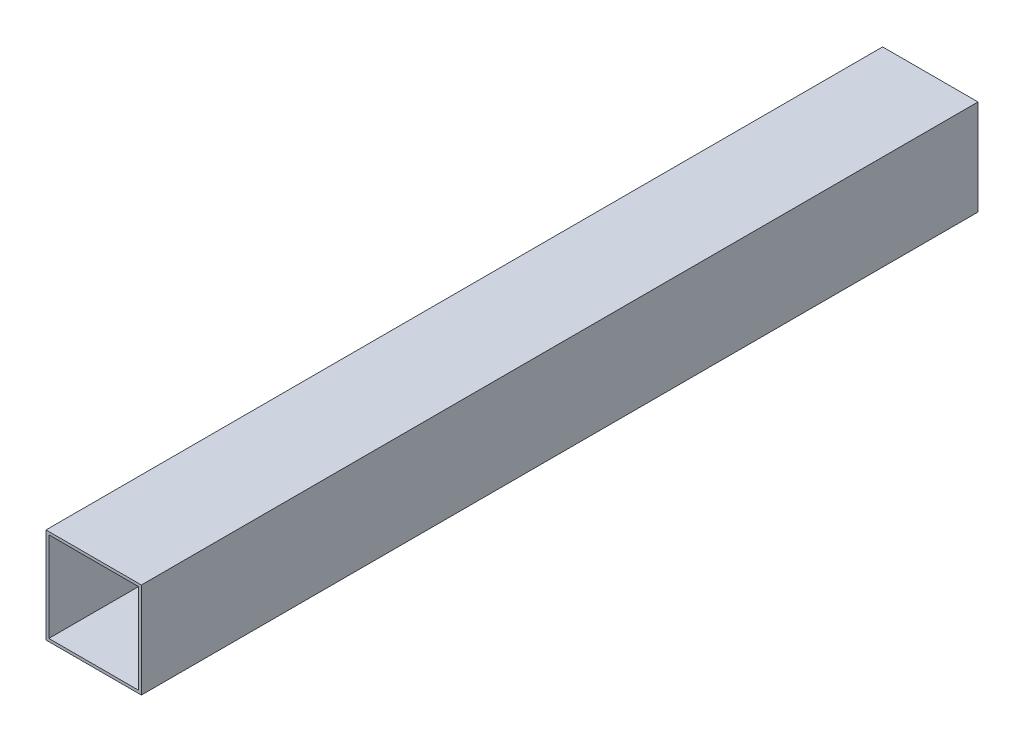
ISO-10303-21;
HEADER;
FILE_DESCRIPTION(('STEP AP214'),'2;1');
FILE_NAME('part.step','',(''),(''),'','','');
FILE_SCHEMA(('AUTOMOTIVE_DESIGN { 1 0 10303 214 1 1 1 1 }'));
ENDSEC;
DATA;
#1=APPLICATION_CONTEXT('core data for automotive mechanical design processes');
#2=APPLICATION_PROTOCOL_DEFINITION('international standard','automotive_design',2000,#1);
#3=PRODUCT_CONTEXT('',#1,'mechanical');
#4=PRODUCT('Part','Part','',(#3));
#5=PRODUCT_RELATED_PRODUCT_CATEGORY('part','',(#4));
#6=PRODUCT_DEFINITION_FORMATION('','',#4);
#7=PRODUCT_DEFINITION_CONTEXT('part definition',#1,'design');
#8=PRODUCT_DEFINITION('design','',#6,#7);
#9=PRODUCT_DEFINITION_SHAPE('','',#8);
#10=(LENGTH_UNIT() NAMED_UNIT(*) SI_UNIT(.MILLI.,.METRE.));
#11=(NAMED_UNIT(*) PLANE_ANGLE_UNIT() SI_UNIT($,.RADIAN.));
#12=(NAMED_UNIT(*) SI_UNIT($,.STERADIAN.) SOLID_ANGLE_UNIT());
#13=UNCERTAINTY_MEASURE_WITH_UNIT(LENGTH_MEASURE(1.E-05),#10,'distance_accuracy_value','');
#14=(GEOMETRIC_REPRESENTATION_CONTEXT(3) GLOBAL_UNCERTAINTY_ASSIGNED_CONTEXT((#13)) GLOBAL_UNIT_ASSIGNED_CONTEXT((#10,
#11,#12)) REPRESENTATION_CONTEXT('',''));
#15=CARTESIAN_POINT('',(0.,0.,0.));
#16=DIRECTION('',(0.,0.,1.));
#17=DIRECTION('',(1.,0.,0.));
#18=AXIS2_PLACEMENT_3D('',#15,#16,#17);
#19=CARTESIAN_POINT('',(0.,107.95,1893.8875));
#20=DIRECTION('',(0.,1.,0.));
#21=DIRECTION('',(0.,0.,1.));
#22=AXIS2_PLACEMENT_3D('',#19,#20,#21);
#23=PLANE('',#22);
#24=DIRECTION('',(1.,0.,0.));
#25=VECTOR('',#24,1.);
#26=CARTESIAN_POINT('',(0.,107.95,0.));
#27=LINE('',#26,#25);
#28=CARTESIAN_POINT('',(-107.95,107.95,0.));
#29=VERTEX_POINT('',#28);
#30=CARTESIAN_POINT('',(107.95,107.95,0.));
#31=VERTEX_POINT('',#30);
#32=EDGE_CURVE('E159',#29,#31,#27,.T.);
#33=ORIENTED_EDGE('',*,*,#32,.F.);
#34=DIRECTION('',(0.,0.,-1.));
#35=VECTOR('',#34,1.);
#36=CARTESIAN_POINT('',(-107.95,107.95,1893.8875));
#37=LINE('',#36,#35);
#38=CARTESIAN_POINT('',(-107.95,107.95,1893.8875));
#39=VERTEX_POINT('',#38);
#40=EDGE_CURVE('E12',#39,#29,#37,.T.);
#41=ORIENTED_EDGE('',*,*,#40,.F.);
#42=DIRECTION('',(1.,0.,0.));
#43=VECTOR('',#42,1.);
#44=CARTESIAN_POINT('',(0.,107.95,1893.8875));
#45=LINE('',#44,#43);
#46=CARTESIAN_POINT('',(107.95,107.95,1893.8875));
#47=VERTEX_POINT('',#46);
#48=EDGE_CURVE('E161',#39,#47,#45,.T.);
#49=ORIENTED_EDGE('',*,*,#48,.T.);
#50=DIRECTION('',(0.,0.,-1.));
#51=VECTOR('',#50,1.);
#52=CARTESIAN_POINT('',(107.95,107.95,1893.8875));
#53=LINE('',#52,#51);
#54=EDGE_CURVE('E67',#47,#31,#53,.T.);
#55=ORIENTED_EDGE('',*,*,#54,.T.);
#56=EDGE_LOOP('',(#33,#41,#49,#55));
#57=FACE_BOUND('',#56,.T.);
#58=ADVANCED_FACE('F61',(#57),#23,.T.);
#59=CARTESIAN_POINT('',(-107.95,0.,1893.8875));
#60=DIRECTION('',(1.,0.,0.));
#61=DIRECTION('',(0.,0.,-1.));
#62=AXIS2_PLACEMENT_3D('',#59,#60,#61);
#63=PLANE('',#62);
#64=DIRECTION('',(0.,-1.,0.));
#65=VECTOR('',#64,1.);
#66=CARTESIAN_POINT('',(-107.95,0.,0.));
#67=LINE('',#66,#65);
#68=CARTESIAN_POINT('',(-107.95,-107.95,0.));
#69=VERTEX_POINT('',#68);
#70=EDGE_CURVE('E167',#29,#69,#67,.T.);
#71=ORIENTED_EDGE('',*,*,#70,.T.);
#72=DIRECTION('',(0.,0.,-1.));
#73=VECTOR('',#72,1.);
#74=CARTESIAN_POINT('',(-107.95,-107.95,1893.8875));
#75=LINE('',#74,#73);
#76=CARTESIAN_POINT('',(-107.95,-107.95,1893.8875));
#77=VERTEX_POINT('',#76);
#78=EDGE_CURVE('E73',#77,#69,#75,.T.);
#79=ORIENTED_EDGE('',*,*,#78,.F.);
#80=DIRECTION('',(0.,-1.,0.));
#81=VECTOR('',#80,1.);
#82=CARTESIAN_POINT('',(-107.95,0.,1893.8875));
#83=LINE('',#82,#81);
#84=EDGE_CURVE('E175',#39,#77,#83,.T.);
#85=ORIENTED_EDGE('',*,*,#84,.F.);
#86=ORIENTED_EDGE('',*,*,#40,.T.);
#87=EDGE_LOOP('',(#71,#79,#85,#86));
#88=FACE_BOUND('',#87,.T.);
#89=ADVANCED_FACE('F197',(#88),#63,.F.);
#90=CARTESIAN_POINT('',(0.,-107.95,1893.8875));
#91=DIRECTION('',(0.,1.,0.));
#92=DIRECTION('',(0.,0.,1.));
#93=AXIS2_PLACEMENT_3D('',#90,#91,#92);
#94=PLANE('',#93);
#95=DIRECTION('',(1.,0.,0.));
#96=VECTOR('',#95,1.);
#97=CARTESIAN_POINT('',(0.,-107.95,0.));
#98=LINE('',#97,#96);
#99=CARTESIAN_POINT('',(107.95,-107.95,0.));
#100=VERTEX_POINT('',#99);
#101=EDGE_CURVE('E177',#69,#100,#98,.T.);
#102=ORIENTED_EDGE('',*,*,#101,.T.);
#103=DIRECTION('',(0.,0.,-1.));
#104=VECTOR('',#103,1.);
#105=CARTESIAN_POINT('',(107.95,-107.95,1893.8875));
#106=LINE('',#105,#104);
#107=CARTESIAN_POINT('',(107.95,-107.95,1893.8875));
#108=VERTEX_POINT('',#107);
#109=EDGE_CURVE('E182',#108,#100,#106,.T.);
#110=ORIENTED_EDGE('',*,*,#109,.F.);
#111=DIRECTION('',(1.,0.,0.));
#112=VECTOR('',#111,1.);
#113=CARTESIAN_POINT('',(0.,-107.95,1893.8875));
#114=LINE('',#113,#112);
#115=EDGE_CURVE('E169',#77,#108,#114,.T.);
#116=ORIENTED_EDGE('',*,*,#115,.F.);
#117=ORIENTED_EDGE('',*,*,#78,.T.);
#118=EDGE_LOOP('',(#102,#110,#116,#117));
#119=FACE_BOUND('',#118,.T.);
#120=ADVANCED_FACE('F201',(#119),#94,.F.);
#121=CARTESIAN_POINT('',(107.95,0.,1893.8875));
#122=DIRECTION('',(1.,0.,0.));
#123=DIRECTION('',(0.,1.,0.));
#124=AXIS2_PLACEMENT_3D('',#121,#122,#123);
#125=PLANE('',#124);
#126=DIRECTION('',(0.,-1.,0.));
#127=VECTOR('',#126,1.);
#128=CARTESIAN_POINT('',(107.95,0.,0.));
#129=LINE('',#128,#127);
#130=EDGE_CURVE('E176',#31,#100,#129,.T.);
#131=ORIENTED_EDGE('',*,*,#130,.F.);
#132=ORIENTED_EDGE('',*,*,#54,.F.);
#133=DIRECTION('',(0.,-1.,0.));
#134=VECTOR('',#133,1.);
#135=CARTESIAN_POINT('',(107.95,0.,1893.8875));
#136=LINE('',#135,#134);
#137=EDGE_CURVE('E168',#47,#108,#136,.T.);
#138=ORIENTED_EDGE('',*,*,#137,.T.);
#139=ORIENTED_EDGE('',*,*,#109,.T.);
#140=EDGE_LOOP('',(#131,#132,#138,#139));
#141=FACE_BOUND('',#140,.T.);
#142=ADVANCED_FACE('F195',(#141),#125,.T.);
#143=CARTESIAN_POINT('',(0.,0.,1893.8875));
#144=DIRECTION('',(0.,0.,-1.));
#145=DIRECTION('',(-1.,0.,0.));
#146=AXIS2_PLACEMENT_3D('',#143,#144,#145);
#147=PLANE('',#146);
#148=DIRECTION('',(0.,-1.,0.));
#149=VECTOR('',#148,1.);
#150=CARTESIAN_POINT('',(-101.6,101.6,1893.8875));
#151=LINE('',#150,#149);
#152=CARTESIAN_POINT('',(-101.6,101.6,1893.8875));
#153=VERTEX_POINT('',#152);
#154=CARTESIAN_POINT('',(-101.6,-101.6,1893.8875));
#155=VERTEX_POINT('',#154);
#156=EDGE_CURVE('E133',#153,#155,#151,.T.);
#157=ORIENTED_EDGE('',*,*,#156,.F.);
#158=DIRECTION('',(1.,0.,0.));
#159=VECTOR('',#158,1.);
#160=CARTESIAN_POINT('',(-101.6,101.6,1893.8875));
#161=LINE('',#160,#159);
#162=CARTESIAN_POINT('',(101.6,101.6,1893.8875));
#163=VERTEX_POINT('',#162);
#164=EDGE_CURVE('E127',#153,#163,#161,.T.);
#165=ORIENTED_EDGE('',*,*,#164,.T.);
#166=DIRECTION('',(0.,-1.,0.));
#167=VECTOR('',#166,1.);
#168=CARTESIAN_POINT('',(101.6,101.6,1893.8875));
#169=LINE('',#168,#167);
#170=CARTESIAN_POINT('',(101.6,-101.6,1893.8875));
#171=VERTEX_POINT('',#170);
#172=EDGE_CURVE('E136',#163,#171,#169,.T.);
#173=ORIENTED_EDGE('',*,*,#172,.T.);
#174=DIRECTION('',(1.,0.,0.));
#175=VECTOR('',#174,1.);
#176=CARTESIAN_POINT('',(-101.6,-101.6,1893.8875));
#177=LINE('',#176,#175);
#178=EDGE_CURVE('E139',#155,#171,#177,.T.);
#179=ORIENTED_EDGE('',*,*,#178,.F.);
#180=EDGE_LOOP('',(#157,#165,#173,#179));
#181=FACE_BOUND('',#180,.T.);
#182=ORIENTED_EDGE('',*,*,#48,.F.);
#183=ORIENTED_EDGE('',*,*,#84,.T.);
#184=ORIENTED_EDGE('',*,*,#115,.T.);
#185=ORIENTED_EDGE('',*,*,#137,.F.);
#186=EDGE_LOOP('',(#182,#183,#184,#185));
#187=FACE_BOUND('',#186,.T.);
#188=ADVANCED_FACE('F145',(#181,#187),#147,.F.);
#189=CARTESIAN_POINT('',(0.,0.,0.));
#190=DIRECTION('',(0.,0.,-1.));
#191=DIRECTION('',(-1.,0.,0.));
#192=AXIS2_PLACEMENT_3D('',#189,#190,#191);
#193=PLANE('',#192);
#194=DIRECTION('',(1.,0.,0.));
#195=VECTOR('',#194,1.);
#196=CARTESIAN_POINT('',(-101.6,101.6,0.));
#197=LINE('',#196,#195);
#198=CARTESIAN_POINT('',(-101.6,101.6,0.));
#199=VERTEX_POINT('',#198);
#200=CARTESIAN_POINT('',(101.6,101.6,0.));
#201=VERTEX_POINT('',#200);
#202=EDGE_CURVE('E90',#199,#201,#197,.T.);
#203=ORIENTED_EDGE('',*,*,#202,.F.);
#204=DIRECTION('',(0.,-1.,0.));
#205=VECTOR('',#204,1.);
#206=CARTESIAN_POINT('',(-101.6,101.6,0.));
#207=LINE('',#206,#205);
#208=CARTESIAN_POINT('',(-101.6,-101.6,0.));
#209=VERTEX_POINT('',#208);
#210=EDGE_CURVE('E143',#199,#209,#207,.T.);
#211=ORIENTED_EDGE('',*,*,#210,.T.);
#212=DIRECTION('',(1.,0.,0.));
#213=VECTOR('',#212,1.);
#214=CARTESIAN_POINT('',(-101.6,-101.6,0.));
#215=LINE('',#214,#213);
#216=CARTESIAN_POINT('',(101.6,-101.6,0.));
#217=VERTEX_POINT('',#216);
#218=EDGE_CURVE('E150',#209,#217,#215,.T.);
#219=ORIENTED_EDGE('',*,*,#218,.T.);
#220=DIRECTION('',(0.,-1.,0.));
#221=VECTOR('',#220,1.);
#222=CARTESIAN_POINT('',(101.6,101.6,0.));
#223=LINE('',#222,#221);
#224=EDGE_CURVE('E151',#201,#217,#223,.T.);
#225=ORIENTED_EDGE('',*,*,#224,.F.);
#226=EDGE_LOOP('',(#203,#211,#219,#225));
#227=FACE_BOUND('',#226,.T.);
#228=ORIENTED_EDGE('',*,*,#32,.T.);
#229=ORIENTED_EDGE('',*,*,#130,.T.);
#230=ORIENTED_EDGE('',*,*,#101,.F.);
#231=ORIENTED_EDGE('',*,*,#70,.F.);
#232=EDGE_LOOP('',(#228,#229,#230,#231));
#233=FACE_BOUND('',#232,.T.);
#234=ADVANCED_FACE('F198',(#227,#233),#193,.T.);
#235=CARTESIAN_POINT('',(-101.6,101.6,1893.8875));
#236=DIRECTION('',(0.,1.,0.));
#237=DIRECTION('',(0.,0.,1.));
#238=AXIS2_PLACEMENT_3D('',#235,#236,#237);
#239=PLANE('',#238);
#240=ORIENTED_EDGE('',*,*,#202,.T.);
#241=DIRECTION('',(0.,0.,-1.));
#242=VECTOR('',#241,1.);
#243=CARTESIAN_POINT('',(101.6,101.6,1893.8875));
#244=LINE('',#243,#242);
#245=EDGE_CURVE('E130',#163,#201,#244,.T.);
#246=ORIENTED_EDGE('',*,*,#245,.F.);
#247=ORIENTED_EDGE('',*,*,#164,.F.);
#248=DIRECTION('',(0.,0.,-1.));
#249=VECTOR('',#248,1.);
#250=CARTESIAN_POINT('',(-101.6,101.6,1893.8875));
#251=LINE('',#250,#249);
#252=EDGE_CURVE('E160',#153,#199,#251,.T.);
#253=ORIENTED_EDGE('',*,*,#252,.T.);
#254=EDGE_LOOP('',(#240,#246,#247,#253));
#255=FACE_BOUND('',#254,.T.);
#256=ADVANCED_FACE('F126',(#255),#239,.F.);
#257=CARTESIAN_POINT('',(-101.6,101.6,1893.8875));
#258=DIRECTION('',(1.,0.,0.));
#259=DIRECTION('',(0.,0.,-1.));
#260=AXIS2_PLACEMENT_3D('',#257,#258,#259);
#261=PLANE('',#260);
#262=ORIENTED_EDGE('',*,*,#210,.F.);
#263=ORIENTED_EDGE('',*,*,#252,.F.);
#264=ORIENTED_EDGE('',*,*,#156,.T.);
#265=DIRECTION('',(0.,0.,-1.));
#266=VECTOR('',#265,1.);
#267=CARTESIAN_POINT('',(-101.6,-101.6,1893.8875));
#268=LINE('',#267,#266);
#269=EDGE_CURVE('E158',#155,#209,#268,.T.);
#270=ORIENTED_EDGE('',*,*,#269,.T.);
#271=EDGE_LOOP('',(#262,#263,#264,#270));
#272=FACE_BOUND('',#271,.T.);
#273=ADVANCED_FACE('F249',(#272),#261,.T.);
#274=CARTESIAN_POINT('',(-101.6,-101.6,1893.8875));
#275=DIRECTION('',(0.,1.,0.));
#276=DIRECTION('',(0.,0.,1.));
#277=AXIS2_PLACEMENT_3D('',#274,#275,#276);
#278=PLANE('',#277);
#279=ORIENTED_EDGE('',*,*,#218,.F.);
#280=ORIENTED_EDGE('',*,*,#269,.F.);
#281=ORIENTED_EDGE('',*,*,#178,.T.);
#282=DIRECTION('',(0.,0.,-1.));
#283=VECTOR('',#282,1.);
#284=CARTESIAN_POINT('',(101.6,-101.6,1893.8875));
#285=LINE('',#284,#283);
#286=EDGE_CURVE('E80',#171,#217,#285,.T.);
#287=ORIENTED_EDGE('',*,*,#286,.T.);
#288=EDGE_LOOP('',(#279,#280,#281,#287));
#289=FACE_BOUND('',#288,.T.);
#290=ADVANCED_FACE('F257',(#289),#278,.T.);
#291=CARTESIAN_POINT('',(101.6,101.6,1893.8875));
#292=DIRECTION('',(1.,0.,0.));
#293=DIRECTION('',(0.,1.,0.));
#294=AXIS2_PLACEMENT_3D('',#291,#292,#293);
#295=PLANE('',#294);
#296=ORIENTED_EDGE('',*,*,#224,.T.);
#297=ORIENTED_EDGE('',*,*,#286,.F.);
#298=ORIENTED_EDGE('',*,*,#172,.F.);
#299=ORIENTED_EDGE('',*,*,#245,.T.);
#300=EDGE_LOOP('',(#296,#297,#298,#299));
#301=FACE_BOUND('',#300,.T.);
#302=ADVANCED_FACE('F140',(#301),#295,.F.);
#303=CLOSED_SHELL('',(#58,#89,#120,#142,#188,#234,#256,#273,#290,#302));
#304=MANIFOLD_SOLID_BREP('B2',#303);
#305=ADVANCED_BREP_SHAPE_REPRESENTATION('',(#18,#304),#14);
#306=SHAPE_DEFINITION_REPRESENTATION(#9,#305);
ENDSEC;
END-ISO-10303-21;
